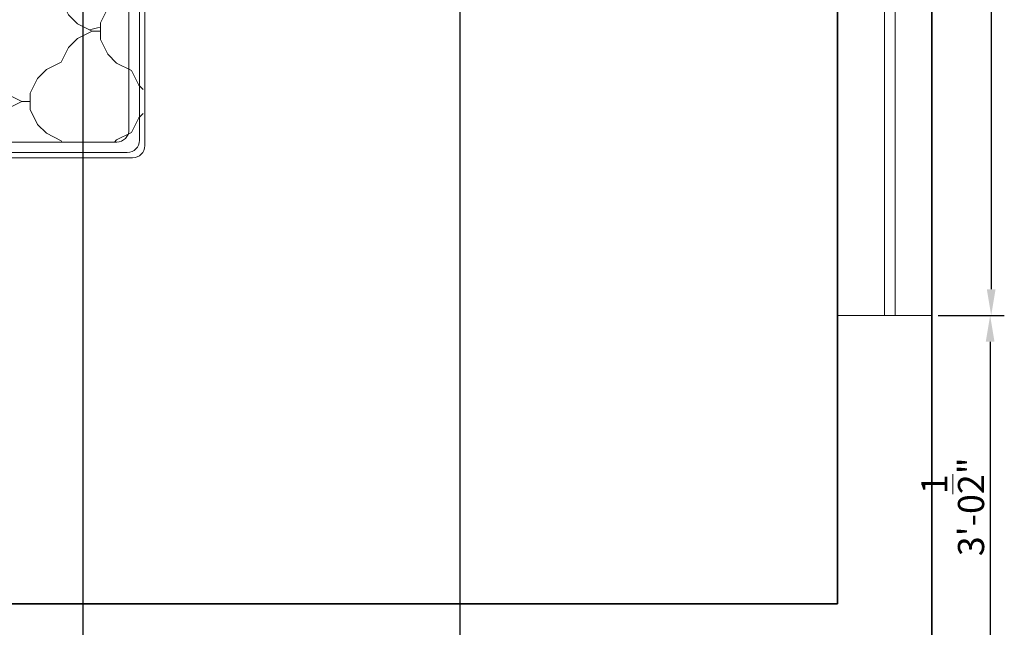
# Model space of a CAD drawing. Units: inches. Extents: x 1624 to 3956, y 1589 to 5028.
# Tile 5 of 16: x 2014 to 2108, y 2075 to 2133. Entities that reach past the tile are written whole.
import ezdxf

# ---------------------------------------------------------------- set-up
doc = ezdxf.new("R2010")
doc.units = ezdxf.units.IN
for name, color, linetype, lineweight in [('A-ANNO-DIMS', 2, 'Continuous', 13), ('A-FURN', 8, 'Continuous', 18), ('A-GLAZ', 4, 'Continuous', 18), ('A-WALL', 7, 'Continuous', 35)]:
    doc.layers.add(name, color=color, linetype=linetype, lineweight=lineweight)
doc.styles.get("Standard").update_dxf_attribs({"font": 'arial.ttf'})
doc.dimstyles.new('Copy of ISO-25', dxfattribs={"dimtxt": 2.5, "dimasz": 2.5, "dimexe": 1.25, "dimexo": 0.625, "dimtad": 1, "dimdec": 1, "dimlunit": 4, "dimtxsty": 'Standard', "dimcen": 2.5, "dimadec": 0, "dimazin": 0, "dimtfac": 1, "dimtdec": 1, "dimtmove": 0, "dimatfit": 3, "dimfxl": 1, "dimarcsym": 0})

# ---------------------------------------------------------------- blocks, each defined once
blk = doc.blocks.new('A$C029D5C69')
for p, q in [((0.4164, 2.0693), (0.4164, 2.0066)), ((2.2315, 2.0693), (0.4164, 2.0693)), ((2.2315, 2.0066), (2.2315, 2.0693)), ((0, 1.606), (0, 2.0066)), ((0, 2.0066), (0.505, 2.0066)), ((0.4164, 2.0066), (2.2315, 2.0066)), ((0.505, 2.0066), (0.505, 1.606)), ((0.5252, 0.0351), (0.5252, 2.0066)), ((0.5403, 0.0502), (0.5403, 2.0066)), ((0.5706, 0.0805), (0.5706, 2.0066)), ((0.6869, 1.966), (0.6666, 2.0066)), ((0.7072, 2.0066), (0.6869, 1.966)), ((1.0902, 1.966), (1.0699, 2.0066)), ((1.1106, 2.0066), (1.0902, 1.966)), ((2.1114, 2.0087), (2.1114, 0.0351)), ((2.6479, 2.0066), (2.1429, 2.0066)), ((2.1429, 2.0066), (2.1429, 1.606)), ((2.6479, 1.606), (2.6479, 2.0066)), ((0.0151, 1.6211), (0.0151, 1.9915)), ((0.0151, 1.9915), (0.4899, 1.9915)), ((0.4899, 1.9915), (0.4899, 1.6211)), ((1.8954, 1.9865), (1.3081, 1.9865)), ((2.6328, 1.9915), (2.158, 1.9915)), ((2.158, 1.9915), (2.158, 1.6211)), ((2.6328, 1.6211), (2.6328, 1.9915)), ((0.2689, 1.9609), (0.2689, 1.6764)), ((0.6869, 1.9425), (0.6869, 1.966)), ((0.6869, 1.9425), (0.6869, 1.966)), ((1.0902, 1.9425), (1.0902, 1.966)), ((1.0902, 1.9425), (1.0902, 1.966)), ((1.8954, 1.9713), (1.3339, 1.9713)), ((1.3849, 1.9713), (1.3656, 1.952)), ((1.3945, 1.9713), (1.3714, 1.9483)), ((1.4249, 1.945), (1.3986, 1.9713)), ((1.4288, 1.9507), (1.4081, 1.9713)), ((1.4476, 1.9507), (1.4288, 1.9507)), ((1.4476, 1.9507), (1.4664, 1.9507)), ((1.487, 1.9713), (1.4664, 1.9507)), ((1.4966, 1.9713), (1.4703, 1.945)), ((1.527, 1.945), (1.5007, 1.9713)), ((1.5309, 1.9507), (1.5102, 1.9713)), ((1.5497, 1.9507), (1.5309, 1.9507)), ((1.5497, 1.9507), (1.5685, 1.9507)), ((1.5891, 1.9713), (1.5685, 1.9507)), ((1.5987, 1.9713), (1.5724, 1.945)), ((1.6291, 1.945), (1.6028, 1.9713)), ((1.633, 1.9507), (1.6123, 1.9713)), ((1.6518, 1.9507), (1.633, 1.9507)), ((1.6518, 1.9507), (1.6706, 1.9507)), ((1.6912, 1.9713), (1.6706, 1.9507)), ((1.7008, 1.9713), (1.6745, 1.945)), ((1.7312, 1.945), (1.7049, 1.9713)), ((1.7351, 1.9507), (1.7144, 1.9713)), ((1.7539, 1.9507), (1.7351, 1.9507)), ((1.7539, 1.9507), (1.7727, 1.9507)), ((1.7933, 1.9713), (1.7727, 1.9507)), ((1.8029, 1.9713), (1.7766, 1.945)), ((1.8333, 1.945), (1.807, 1.9713)), ((1.8372, 1.9507), (1.8165, 1.9713)), ((1.856, 1.9507), (1.8372, 1.9507)), ((1.856, 1.9507), (1.8748, 1.9507)), ((1.8954, 1.9713), (1.8748, 1.9507)), ((1.9043, 1.9707), (1.8787, 1.945)), ((1.9354, 1.945), (1.9114, 1.969)), ((2.379, 1.9609), (2.379, 1.6764)), ((0.6634, 1.9425), (0.621, 1.9213)), ((0.6634, 1.9425), (0.621, 1.9213)), ((0.6869, 1.9425), (0.6634, 1.9425)), ((0.6869, 1.9425), (0.7104, 1.9425)), ((0.7528, 1.9213), (0.7104, 1.9425)), ((0.7528, 1.9213), (0.7104, 1.9425)), ((1.0668, 1.9425), (1.0244, 1.9213)), ((1.0668, 1.9425), (1.0244, 1.9213)), ((1.0902, 1.9425), (1.0668, 1.9425)), ((1.0902, 1.9425), (1.1137, 1.9425)), ((1.1561, 1.9213), (1.1137, 1.9425)), ((1.1561, 1.9213), (1.1137, 1.9425)), ((1.4249, 1.945), (1.4059, 1.926)), ((1.4288, 1.9394), (1.4116, 1.9222)), ((1.4288, 1.9393), (1.4476, 1.9393)), ((1.4664, 1.9393), (1.4476, 1.9393)), ((1.493, 1.9128), (1.4664, 1.9394)), ((1.4986, 1.9167), (1.4703, 1.945)), ((1.527, 1.945), (1.4986, 1.9167)), ((1.5309, 1.9394), (1.5043, 1.9128)), ((1.5309, 1.9393), (1.5497, 1.9393)), ((1.5685, 1.9393), (1.5497, 1.9393)), ((1.595, 1.9128), (1.5685, 1.9394)), ((1.6007, 1.9167), (1.5724, 1.945)), ((1.6291, 1.945), (1.6007, 1.9167)), ((1.633, 1.9394), (1.6064, 1.9128)), ((1.633, 1.9393), (1.6518, 1.9393)), ((1.6706, 1.9393), (1.6518, 1.9393)), ((1.6971, 1.9128), (1.6706, 1.9394)), ((1.7028, 1.9167), (1.6745, 1.945)), ((1.7312, 1.945), (1.7028, 1.9167)), ((1.7351, 1.9394), (1.7085, 1.9128)), ((1.7351, 1.9393), (1.7539, 1.9393)), ((1.7727, 1.9393), (1.7539, 1.9393)), ((1.7992, 1.9128), (1.7727, 1.9394)), ((1.8049, 1.9167), (1.7766, 1.945)), ((1.8333, 1.945), (1.8049, 1.9167)), ((1.8372, 1.9394), (1.8106, 1.9128)), ((1.8372, 1.9393), (1.856, 1.9393)), ((1.8748, 1.9393), (1.856, 1.9393)), ((1.9013, 1.9128), (1.8748, 1.9394)), ((1.907, 1.9167), (1.8787, 1.945)), ((1.9354, 1.945), (1.907, 1.9167)), ((1.9393, 1.9394), (1.9127, 1.9128)), ((1.9393, 1.9393), (1.9404, 1.9393)), ((1.9414, 1.688), (1.9414, 1.931)), ((1.9565, 1.688), (1.9565, 1.931)), ((0.5955, 1.8958), (0.5743, 1.8534)), ((0.621, 1.9213), (0.5955, 1.8958)), ((0.7783, 1.8958), (0.7528, 1.9213)), ((0.7995, 1.8534), (0.7783, 1.8958)), ((0.9989, 1.8958), (0.9777, 1.8534)), ((1.0243, 1.9213), (0.9988, 1.8958)), ((1.1816, 1.8958), (1.1561, 1.9213)), ((1.2028, 1.8534), (1.1816, 1.8958)), ((1.493, 1.8752), (1.493, 1.9128)), ((1.5043, 1.8752), (1.5043, 1.9128)), ((1.595, 1.8752), (1.595, 1.9128)), ((1.6064, 1.8752), (1.6064, 1.9128)), ((1.6971, 1.8752), (1.6971, 1.9128)), ((1.7085, 1.8752), (1.7085, 1.9128)), ((1.7992, 1.8752), (1.7992, 1.9128)), ((1.8106, 1.8752), (1.8106, 1.9128)), ((1.9013, 1.8752), (1.9013, 1.9128)), ((1.9127, 1.8752), (1.9127, 1.9128)), ((1.493, 1.8752), (1.4867, 1.869)), ((1.4986, 1.8713), (1.4922, 1.8648)), ((1.527, 1.8429), (1.4986, 1.8713)), ((1.5309, 1.8486), (1.5043, 1.8752)), ((1.595, 1.8752), (1.5685, 1.8486)), ((1.6007, 1.8713), (1.5724, 1.8429)), ((1.6291, 1.8429), (1.6007, 1.8713)), ((1.633, 1.8486), (1.6064, 1.8752)), ((1.6971, 1.8752), (1.6706, 1.8486)), ((1.7028, 1.8713), (1.6745, 1.8429)), ((1.7312, 1.8429), (1.7028, 1.8713)), ((1.7351, 1.8486), (1.7085, 1.8752)), ((1.7992, 1.8752), (1.7727, 1.8486)), ((1.8049, 1.8713), (1.7766, 1.8429)), ((1.8333, 1.8429), (1.8049, 1.8713)), ((1.8372, 1.8486), (1.8106, 1.8752)), ((1.9013, 1.8752), (1.8748, 1.8486)), ((1.907, 1.8713), (1.8787, 1.8429)), ((1.9354, 1.8429), (1.907, 1.8713)), ((1.9393, 1.8486), (1.9127, 1.8752)), ((0.5743, 1.8534), (0.5706, 1.8515)), ((0.5743, 1.8534), (0.5706, 1.8515)), ((0.8419, 1.8322), (0.7995, 1.8534)), ((0.8419, 1.8322), (0.7995, 1.8534)), ((0.9777, 1.8534), (0.9353, 1.8322)), ((0.9777, 1.8534), (0.9353, 1.8322)), ((1.2452, 1.8322), (1.2028, 1.8534)), ((1.2452, 1.8322), (1.2028, 1.8534)), ((1.527, 1.8429), (1.5242, 1.8401)), ((1.5309, 1.8373), (1.5295, 1.8359)), ((1.5497, 1.8486), (1.5309, 1.8486)), ((1.5309, 1.8373), (1.5497, 1.8373)), ((1.5497, 1.8486), (1.5685, 1.8486)), ((1.5685, 1.8373), (1.5497, 1.8373)), ((1.595, 1.8107), (1.5685, 1.8373)), ((1.6007, 1.8146), (1.5724, 1.8429)), ((1.6291, 1.8429), (1.6007, 1.8146)), ((1.633, 1.8373), (1.6064, 1.8107)), ((1.6518, 1.8486), (1.633, 1.8486)), ((1.633, 1.8373), (1.6518, 1.8373)), ((1.6518, 1.8486), (1.6706, 1.8486)), ((1.6706, 1.8373), (1.6518, 1.8373)), ((1.6971, 1.8107), (1.6706, 1.8373)), ((1.7028, 1.8146), (1.6745, 1.8429)), ((1.7312, 1.8429), (1.7028, 1.8146)), ((1.7351, 1.8373), (1.7085, 1.8107)), ((1.7539, 1.8486), (1.7351, 1.8486)), ((1.7351, 1.8373), (1.7539, 1.8373)), ((1.7539, 1.8486), (1.7727, 1.8486)), ((1.7727, 1.8373), (1.7539, 1.8373)), ((1.7992, 1.8107), (1.7727, 1.8373)), ((1.8049, 1.8146), (1.7766, 1.8429)), ((1.8333, 1.8429), (1.8049, 1.8146)), ((1.8372, 1.8373), (1.8106, 1.8107)), ((1.856, 1.8486), (1.8372, 1.8486)), ((1.8372, 1.8373), (1.856, 1.8373)), ((1.856, 1.8486), (1.8748, 1.8486)), ((1.8748, 1.8373), (1.856, 1.8373)), ((1.9013, 1.8107), (1.8748, 1.8373)), ((1.907, 1.8146), (1.8787, 1.8429)), ((1.9354, 1.8429), (1.907, 1.8146)), ((1.9393, 1.8373), (1.9127, 1.8107)), ((1.9414, 1.8486), (1.9393, 1.8486)), ((1.9393, 1.8373), (1.9414, 1.8373)), ((0.1267, 1.8186), (0.4111, 1.8186)), ((0.8674, 1.8067), (0.8419, 1.8322)), ((0.9352, 1.8322), (0.9097, 1.8067)), ((1.2707, 1.8067), (1.2452, 1.8322)), ((1.595, 1.7806), (1.595, 1.8107)), ((1.6064, 1.7731), (1.6064, 1.8107)), ((1.6971, 1.7731), (1.6971, 1.8107)), ((1.7085, 1.7731), (1.7085, 1.8107)), ((1.7992, 1.7731), (1.7992, 1.8107)), ((1.8106, 1.7731), (1.8106, 1.8107)), ((1.9013, 1.7731), (1.9013, 1.8107)), ((1.9127, 1.7731), (1.9127, 1.8107)), ((2.2367, 1.8186), (2.5212, 1.8186)), ((0.8886, 1.7643), (0.8674, 1.8067)), ((0.9098, 1.8067), (0.8886, 1.7643)), ((1.2919, 1.7643), (1.2707, 1.8067)), ((0.8886, 1.7408), (0.8886, 1.7643)), ((1.2981, 1.7768), (1.2919, 1.7643)), ((1.2919, 1.7519), (1.2919, 1.7643)), ((1.633, 1.7465), (1.6064, 1.7731)), ((1.6971, 1.7731), (1.6706, 1.7465)), ((1.7028, 1.7692), (1.6745, 1.7408)), ((1.7312, 1.7408), (1.7028, 1.7692)), ((1.7351, 1.7465), (1.7085, 1.7731)), ((1.7992, 1.7731), (1.7727, 1.7465)), ((1.8049, 1.7692), (1.7766, 1.7408)), ((1.8333, 1.7408), (1.8049, 1.7692)), ((1.8372, 1.7465), (1.8106, 1.7731)), ((1.9013, 1.7731), (1.8748, 1.7465)), ((1.907, 1.7692), (1.8787, 1.7408)), ((1.9354, 1.7408), (1.907, 1.7692)), ((1.9393, 1.7465), (1.9127, 1.7731)), ((0.8651, 1.7408), (0.8227, 1.7196)), ((0.8651, 1.7408), (0.8227, 1.7196)), ((0.912, 1.7408), (0.8651, 1.7408)), ((0.9544, 1.7196), (0.912, 1.7408)), ((0.9544, 1.7196), (0.912, 1.7408)), ((1.2684, 1.7408), (1.226, 1.7196)), ((1.2684, 1.7408), (1.226, 1.7196)), ((1.2885, 1.7408), (1.2684, 1.7408)), ((1.6518, 1.7465), (1.633, 1.7465)), ((1.6443, 1.7352), (1.6518, 1.7352)), ((1.6518, 1.7465), (1.6706, 1.7465)), ((1.6706, 1.7352), (1.6518, 1.7352)), ((1.6971, 1.7086), (1.6706, 1.7352)), ((1.7028, 1.7125), (1.6745, 1.7408)), ((1.7312, 1.7408), (1.7028, 1.7125)), ((1.7351, 1.7352), (1.7085, 1.7086)), ((1.7539, 1.7465), (1.7351, 1.7465)), ((1.7351, 1.7352), (1.7539, 1.7352)), ((1.7539, 1.7465), (1.7727, 1.7465)), ((1.7727, 1.7352), (1.7539, 1.7352)), ((1.7992, 1.7086), (1.7727, 1.7352)), ((1.8049, 1.7125), (1.7766, 1.7408)), ((1.8333, 1.7408), (1.8049, 1.7125)), ((1.8372, 1.7352), (1.8106, 1.7086)), ((1.856, 1.7465), (1.8372, 1.7465)), ((1.8372, 1.7352), (1.856, 1.7352)), ((1.856, 1.7465), (1.8748, 1.7465)), ((1.8748, 1.7352), (1.856, 1.7352)), ((1.9013, 1.7086), (1.8748, 1.7352)), ((1.907, 1.7125), (1.8787, 1.7408)), ((1.9354, 1.7408), (1.907, 1.7125)), ((1.9393, 1.7352), (1.9127, 1.7086)), ((1.9414, 1.7465), (1.9393, 1.7465)), ((1.9393, 1.7352), (1.9414, 1.7352)), ((0.5766, 1.6941), (0.5706, 1.7002)), ((0.8227, 1.7196), (0.7972, 1.6941)), ((0.98, 1.6941), (0.9545, 1.7196)), ((1.226, 1.7196), (1.2005, 1.6941)), ((1.6971, 1.682), (1.6971, 1.7086)), ((1.7085, 1.671), (1.7085, 1.7086)), ((1.7992, 1.671), (1.7992, 1.7086)), ((1.8106, 1.671), (1.8106, 1.7086)), ((1.9013, 1.671), (1.9013, 1.7086)), ((1.9127, 1.671), (1.9127, 1.7086)), ((2.5551, 1.6275), (2.5551, 1.696)), ((0.5978, 1.6517), (0.5766, 1.6941)), ((0.7972, 1.6941), (0.776, 1.6517)), ((1.0011, 1.6517), (0.9799, 1.6941)), ((1.2005, 1.6941), (1.1793, 1.6517)), ((1.7318, 1.6477), (1.7085, 1.671)), ((1.7992, 1.671), (1.7759, 1.6477)), ((1.8339, 1.6477), (1.8106, 1.671)), ((1.9013, 1.671), (1.878, 1.6477)), ((1.926, 1.6577), (1.9127, 1.671)), ((0.6402, 1.6305), (0.5978, 1.6517)), ((0.6402, 1.6305), (0.5978, 1.6517)), ((0.776, 1.6517), (0.7336, 1.6305)), ((0.776, 1.6517), (0.7336, 1.6305)), ((1.0435, 1.6305), (1.0011, 1.6517)), ((1.0435, 1.6305), (1.0011, 1.6517)), ((1.1793, 1.6517), (1.1369, 1.6305)), ((1.1793, 1.6517), (1.1369, 1.6305)), ((1.8961, 1.6477), (1.7289, 1.6477)), ((1.8049, 1.6671), (1.7855, 1.6477)), ((1.8244, 1.6477), (1.8049, 1.6671)), ((1.907, 1.6671), (1.8876, 1.6477)), ((1.9202, 1.6539), (1.907, 1.6671)), ((0.4899, 1.6211), (0.0151, 1.6211)), ((0.6657, 1.605), (0.6402, 1.6305)), ((0.7336, 1.6305), (0.7081, 1.605)), ((1.0691, 1.605), (1.0436, 1.6305)), ((1.1369, 1.6305), (1.1114, 1.605)), ((1.8961, 1.6325), (1.7422, 1.6325)), ((2.158, 1.6211), (2.6328, 1.6211)), ((0.505, 1.606), (0, 1.606)), ((0.6869, 1.5626), (0.6657, 1.605)), ((0.7081, 1.605), (0.6869, 1.5626)), ((1.0902, 1.5626), (1.069, 1.605)), ((1.1114, 1.605), (1.0902, 1.5626)), ((2.1429, 1.606), (2.6479, 1.606)), ((0.6869, 1.5392), (0.6869, 1.5626)), ((0.6869, 1.5392), (0.6869, 1.5626)), ((1.0902, 1.5392), (1.0902, 1.5626)), ((1.0902, 1.5392), (1.0902, 1.5626)), ((0.6634, 1.5391), (0.621, 1.5179)), ((0.6634, 1.5391), (0.621, 1.5179)), ((0.6869, 1.5392), (0.6634, 1.5392)), ((0.6869, 1.5392), (0.7104, 1.5392)), ((0.7528, 1.5179), (0.7104, 1.5391)), ((0.7528, 1.5179), (0.7104, 1.5391)), ((1.0668, 1.5391), (1.0244, 1.5179)), ((1.0668, 1.5391), (1.0244, 1.5179)), ((1.0902, 1.5392), (1.0668, 1.5392)), ((1.0902, 1.5392), (1.1137, 1.5392)), ((1.1561, 1.5179), (1.1137, 1.5391)), ((1.1561, 1.5179), (1.1137, 1.5391)), ((1.4534, 1.5308), (1.4277, 1.5179)), ((1.4534, 1.5308), (1.4277, 1.5179)), ((0.621, 1.5179), (0.5955, 1.4924)), ((0.7783, 1.4924), (0.7528, 1.5179)), ((1.0243, 1.5179), (0.9988, 1.4924)), ((1.1816, 1.4924), (1.1561, 1.5179)), ((1.4277, 1.5179), (1.4022, 1.4924)), ((0.5955, 1.4925), (0.5743, 1.4501)), ((0.7995, 1.4501), (0.7783, 1.4925)), ((0.9989, 1.4925), (0.9777, 1.4501)), ((1.2028, 1.4501), (1.1816, 1.4925)), ((1.4022, 1.4925), (1.381, 1.4501)), ((0.5743, 1.45), (0.5706, 1.4481)), ((0.5743, 1.45), (0.5706, 1.4481)), ((0.8419, 1.4288), (0.7995, 1.45)), ((0.8419, 1.4288), (0.7995, 1.45)), ((0.9777, 1.45), (0.9353, 1.4288)), ((0.9777, 1.45), (0.9353, 1.4288)), ((1.2452, 1.4288), (1.2028, 1.45)), ((1.2452, 1.4288), (1.2028, 1.45)), ((1.381, 1.45), (1.3386, 1.4288)), ((1.381, 1.45), (1.3386, 1.4288)), ((1.6062, 1.4501), (1.5966, 1.4692)), ((1.6486, 1.4288), (1.6062, 1.45)), ((1.6486, 1.4288), (1.6062, 1.45)), ((0.8674, 1.4033), (0.8419, 1.4288)), ((0.9352, 1.4288), (0.9097, 1.4033)), ((1.2707, 1.4033), (1.2452, 1.4288)), ((1.3386, 1.4288), (1.3131, 1.4033)), ((1.6741, 1.4033), (1.6486, 1.4288)), ((0.5403, 1.4117), (0.5706, 1.4117)), ((0.8886, 1.361), (0.8674, 1.4034)), ((0.9098, 1.4034), (0.8886, 1.361)), ((1.2919, 1.361), (1.2707, 1.4034)), ((1.3131, 1.4034), (1.2919, 1.361)), ((1.6953, 1.361), (1.6741, 1.4034)), ((1.714, 1.3984), (1.6953, 1.361)), ((0.8886, 1.3375), (0.8886, 1.3609)), ((1.2919, 1.3375), (1.2919, 1.3609)), ((1.6953, 1.3375), (1.6953, 1.3609)), ((0.8651, 1.3374), (0.8227, 1.3162)), ((0.8651, 1.3374), (0.8227, 1.3162)), ((0.912, 1.3375), (0.8651, 1.3375)), ((0.9544, 1.3162), (0.912, 1.3374)), ((0.9544, 1.3162), (0.912, 1.3374)), ((1.2684, 1.3374), (1.226, 1.3162)), ((1.2684, 1.3374), (1.226, 1.3162)), ((1.3154, 1.3375), (1.2684, 1.3375)), ((1.3578, 1.3162), (1.3154, 1.3374)), ((1.3578, 1.3162), (1.3154, 1.3374)), ((1.6718, 1.3374), (1.6294, 1.3162)), ((1.6718, 1.3374), (1.6294, 1.3162)), ((1.7187, 1.3375), (1.6718, 1.3375)), ((1.7611, 1.3162), (1.7187, 1.3374)), ((1.7611, 1.3162), (1.7187, 1.3374)), ((0.8227, 1.3163), (0.7972, 1.2908)), ((0.98, 1.2908), (0.9545, 1.3163)), ((1.226, 1.3163), (1.2005, 1.2908)), ((1.3833, 1.2908), (1.3578, 1.3163)), ((1.6294, 1.3163), (1.6039, 1.2908)), ((1.7867, 1.2908), (1.7611, 1.3163)), ((0.5766, 1.2908), (0.5706, 1.2968)), ((0.5978, 1.2484), (0.5766, 1.2908)), ((0.7972, 1.2908), (0.776, 1.2484)), ((1.0011, 1.2484), (0.9799, 1.2908)), ((1.2005, 1.2908), (1.1793, 1.2484)), ((1.4045, 1.2484), (1.3833, 1.2908)), ((1.6039, 1.2908), (1.5827, 1.2484)), ((1.8078, 1.2484), (1.7866, 1.2908)), ((0.6402, 1.2271), (0.5978, 1.2483)), ((0.6402, 1.2271), (0.5978, 1.2483)), ((0.776, 1.2483), (0.7336, 1.2271)), ((0.776, 1.2483), (0.7336, 1.2271)), ((1.0435, 1.2271), (1.0011, 1.2483)), ((1.0435, 1.2271), (1.0011, 1.2483)), ((1.1793, 1.2483), (1.1369, 1.2271)), ((1.1793, 1.2483), (1.1369, 1.2271)), ((1.4469, 1.2271), (1.4045, 1.2483)), ((1.4469, 1.2271), (1.4045, 1.2483)), ((1.5827, 1.2483), (1.5403, 1.2271)), ((1.5827, 1.2483), (1.5403, 1.2271)), ((1.8502, 1.2271), (1.8078, 1.2483)), ((1.8502, 1.2271), (1.8078, 1.2483)), ((0.6657, 1.2017), (0.6402, 1.2272)), ((0.7336, 1.2272), (0.7081, 1.2017)), ((1.0691, 1.2017), (1.0436, 1.2272)), ((1.1369, 1.2272), (1.1114, 1.2017)), ((1.4724, 1.2017), (1.4469, 1.2272)), ((1.5403, 1.2272), (1.5148, 1.2017)), ((1.8758, 1.2017), (1.8503, 1.2272)), ((0.5403, 1.21), (0.5706, 1.21)), ((0.6869, 1.1593), (0.6657, 1.2017)), ((0.7081, 1.2017), (0.6869, 1.1593)), ((1.0902, 1.1593), (1.069, 1.2017)), ((1.1114, 1.2017), (1.0902, 1.1593)), ((1.4936, 1.1593), (1.4724, 1.2017)), ((1.5148, 1.2017), (1.4936, 1.1593)), ((1.8969, 1.1593), (1.8757, 1.2017)), ((1.9181, 1.2017), (1.8969, 1.1593)), ((1.9215, 1.2051), (1.9181, 1.2017)), ((0.6869, 1.1358), (0.6869, 1.1593)), ((0.6869, 1.1358), (0.6869, 1.1593)), ((1.0902, 1.1358), (1.0902, 1.1593)), ((1.0902, 1.1358), (1.0902, 1.1593)), ((1.4936, 1.1358), (1.4936, 1.1593)), ((1.4936, 1.1358), (1.4936, 1.1593)), ((1.8969, 1.1358), (1.8969, 1.1593)), ((1.8969, 1.1358), (1.8969, 1.1593)), ((0.6634, 1.1358), (0.621, 1.1146)), ((0.6634, 1.1358), (0.621, 1.1146)), ((0.6869, 1.1358), (0.6634, 1.1358)), ((0.6869, 1.1358), (0.7104, 1.1358)), ((0.7528, 1.1146), (0.7104, 1.1358)), ((0.7528, 1.1146), (0.7104, 1.1358)), ((1.0668, 1.1358), (1.0244, 1.1146)), ((1.0668, 1.1358), (1.0244, 1.1146)), ((1.0902, 1.1358), (1.0668, 1.1358)), ((1.0902, 1.1358), (1.1137, 1.1358)), ((1.1561, 1.1146), (1.1137, 1.1358)), ((1.1561, 1.1146), (1.1137, 1.1358)), ((1.4701, 1.1358), (1.4277, 1.1146)), ((1.4701, 1.1358), (1.4277, 1.1146)), ((1.4936, 1.1358), (1.4701, 1.1358)), ((1.4936, 1.1358), (1.5171, 1.1358)), ((1.5595, 1.1146), (1.5171, 1.1358)), ((1.5595, 1.1146), (1.5171, 1.1358)), ((1.8735, 1.1358), (1.8311, 1.1146)), ((1.8735, 1.1358), (1.8311, 1.1146)), ((1.8969, 1.1358), (1.8735, 1.1358)), ((1.8969, 1.1358), (1.9204, 1.1358)), ((1.9628, 1.1146), (1.9204, 1.1358)), ((1.9628, 1.1146), (1.9204, 1.1358)), ((0.621, 1.1146), (0.5955, 1.0891)), ((0.7783, 1.0891), (0.7528, 1.1146)), ((1.0243, 1.1146), (0.9988, 1.0891)), ((1.1816, 1.0891), (1.1561, 1.1146)), ((1.4277, 1.1146), (1.4022, 1.0891)), ((1.585, 1.0891), (1.5595, 1.1146)), ((1.831, 1.1146), (1.8055, 1.0891)), ((1.9883, 1.0891), (1.9628, 1.1146)), ((0.5955, 1.0891), (0.5743, 1.0467)), ((0.7995, 1.0467), (0.7783, 1.0891)), ((0.9989, 1.0891), (0.9777, 1.0467)), ((1.2028, 1.0467), (1.1816, 1.0891)), ((1.4022, 1.0891), (1.381, 1.0467)), ((1.6062, 1.0467), (1.585, 1.0891)), ((1.8056, 1.0891), (1.7844, 1.0467)), ((2.0095, 1.0467), (1.9883, 1.0891)), ((0.5743, 1.0467), (0.5706, 1.0448)), ((0.5743, 1.0467), (0.5706, 1.0448)), ((0.8419, 1.0255), (0.7995, 1.0467)), ((0.8419, 1.0255), (0.7995, 1.0467)), ((0.9777, 1.0467), (0.9353, 1.0255)), ((0.9777, 1.0467), (0.9353, 1.0255)), ((1.2452, 1.0255), (1.2028, 1.0467)), ((1.2452, 1.0255), (1.2028, 1.0467)), ((1.381, 1.0467), (1.3386, 1.0255)), ((1.381, 1.0467), (1.3386, 1.0255)), ((1.6486, 1.0255), (1.6062, 1.0467)), ((1.6486, 1.0255), (1.6062, 1.0467)), ((1.7844, 1.0467), (1.742, 1.0255)), ((1.7844, 1.0467), (1.742, 1.0255)), ((2.0276, 1.0376), (2.0095, 1.0467)), ((2.0276, 1.0376), (2.0095, 1.0467)), ((0.8674, 1), (0.8419, 1.0255)), ((0.9352, 1.0255), (0.9097, 1)), ((1.2707, 1), (1.2452, 1.0255)), ((1.3386, 1.0255), (1.3131, 1)), ((1.6741, 1), (1.6486, 1.0255)), ((1.7419, 1.0255), (1.7164, 1)), ((0.8886, 0.9576), (0.8674, 1)), ((0.9098, 1), (0.8886, 0.9576)), ((1.2919, 0.9576), (1.2707, 1)), ((1.3131, 1), (1.2919, 0.9576)), ((1.6953, 0.9576), (1.6741, 1)), ((1.7165, 1), (1.6953, 0.9576)), ((0.8651, 0.9341), (0.8227, 0.9129)), ((0.8651, 0.9341), (0.8227, 0.9129)), ((0.912, 0.9341), (0.8651, 0.9341)), ((0.8886, 0.9341), (0.8886, 0.9576)), ((0.9544, 0.9129), (0.912, 0.9341)), ((0.9544, 0.9129), (0.912, 0.9341)), ((1.2684, 0.9341), (1.226, 0.9129)), ((1.2684, 0.9341), (1.226, 0.9129)), ((1.3154, 0.9341), (1.2684, 0.9341)), ((1.2919, 0.9341), (1.2919, 0.9576)), ((1.3578, 0.9129), (1.3154, 0.9341)), ((1.3578, 0.9129), (1.3154, 0.9341)), ((1.6718, 0.9341), (1.6294, 0.9129)), ((1.6718, 0.9341), (1.6294, 0.9129)), ((1.7187, 0.9341), (1.6718, 0.9341)), ((1.6953, 0.9341), (1.6953, 0.9576)), ((1.7611, 0.9129), (1.7187, 0.9341)), ((1.7611, 0.9129), (1.7187, 0.9341)), ((2.066, 0.9457), (2.066, 0.0805)), ((0.8227, 0.9129), (0.7972, 0.8874)), ((0.98, 0.8874), (0.9545, 0.9129)), ((1.226, 0.9129), (1.2005, 0.8874)), ((1.3833, 0.8874), (1.3578, 0.9129)), ((1.6294, 0.9129), (1.6039, 0.8874)), ((1.7867, 0.8874), (1.7611, 0.9129)), ((2.0327, 0.9129), (2.0072, 0.8874)), ((2.066, 0.9295), (2.0327, 0.9129)), ((2.066, 0.9295), (2.0327, 0.9129)), ((0.5766, 0.8874), (0.5706, 0.8935)), ((0.5978, 0.845), (0.5766, 0.8874)), ((0.7972, 0.8874), (0.776, 0.845)), ((1.0011, 0.845), (0.9799, 0.8874)), ((1.2005, 0.8874), (1.1793, 0.845)), ((1.4045, 0.845), (1.3833, 0.8874)), ((1.6039, 0.8874), (1.5827, 0.845)), ((1.8078, 0.845), (1.7866, 0.8874)), ((2.0072, 0.8874), (1.986, 0.845)), ((0.6402, 0.8238), (0.5978, 0.845)), ((0.6402, 0.8238), (0.5978, 0.845)), ((0.6657, 0.7983), (0.6402, 0.8238)), ((0.7336, 0.8238), (0.7081, 0.7983)), ((0.776, 0.845), (0.7336, 0.8238)), ((0.776, 0.845), (0.7336, 0.8238)), ((1.0435, 0.8238), (1.0011, 0.845)), ((1.0435, 0.8238), (1.0011, 0.845)), ((1.0691, 0.7983), (1.0436, 0.8238)), ((1.1369, 0.8238), (1.1114, 0.7983)), ((1.1793, 0.845), (1.1369, 0.8238)), ((1.1793, 0.845), (1.1369, 0.8238)), ((1.4469, 0.8238), (1.4045, 0.845)), ((1.4469, 0.8238), (1.4045, 0.845)), ((1.4724, 0.7983), (1.4469, 0.8238)), ((1.5403, 0.8238), (1.5148, 0.7983)), ((1.5827, 0.845), (1.5403, 0.8238)), ((1.5827, 0.845), (1.5403, 0.8238)), ((1.8502, 0.8238), (1.8078, 0.845)), ((1.8502, 0.8238), (1.8078, 0.845)), ((1.8758, 0.7983), (1.8503, 0.8238)), ((1.9436, 0.8238), (1.9181, 0.7983)), ((1.986, 0.845), (1.9436, 0.8238)), ((1.986, 0.845), (1.9436, 0.8238)), ((2.0962, 0.8369), (2.0962, 0.0502)), ((0.6869, 0.7559), (0.6657, 0.7983)), ((0.7081, 0.7983), (0.6869, 0.7559)), ((1.0902, 0.7559), (1.069, 0.7983)), ((1.1114, 0.7983), (1.0902, 0.7559)), ((1.4936, 0.7559), (1.4724, 0.7983)), ((1.5148, 0.7983), (1.4936, 0.7559)), ((1.8969, 0.7559), (1.8757, 0.7983)), ((1.9181, 0.7983), (1.8969, 0.7559)), ((0.6869, 0.7325), (0.6869, 0.7559)), ((0.6869, 0.7325), (0.6869, 0.7559)), ((1.0902, 0.7325), (1.0902, 0.7559)), ((1.0902, 0.7325), (1.0902, 0.7559)), ((1.2024, 0.7028), (1.2503, 0.7507)), ((1.4936, 0.7325), (1.4936, 0.7559)), ((1.4936, 0.7325), (1.4936, 0.7559)), ((1.8969, 0.7325), (1.8969, 0.7559)), ((1.8969, 0.7325), (1.8969, 0.7559)), ((0.621, 0.7113), (0.5955, 0.6858)), ((0.6634, 0.7324), (0.621, 0.7112)), ((0.6634, 0.7324), (0.621, 0.7112)), ((0.6869, 0.7325), (0.6634, 0.7325)), ((0.6869, 0.7325), (0.7104, 0.7325)), ((0.7528, 0.7112), (0.7104, 0.7324)), ((0.7528, 0.7112), (0.7104, 0.7324)), ((0.7783, 0.6858), (0.7528, 0.7113)), ((1.0243, 0.7113), (0.9988, 0.6858)), ((1.0668, 0.7324), (1.0244, 0.7112)), ((1.0668, 0.7324), (1.0244, 0.7112)), ((1.0902, 0.7325), (1.0668, 0.7325)), ((1.0902, 0.7325), (1.1137, 0.7325)), ((1.1561, 0.7112), (1.1137, 0.7324)), ((1.1561, 0.7112), (1.1137, 0.7324)), ((1.1816, 0.6858), (1.1561, 0.7113)), ((1.4277, 0.7113), (1.4022, 0.6858)), ((1.4701, 0.7324), (1.4277, 0.7112)), ((1.4701, 0.7324), (1.4277, 0.7112)), ((1.4936, 0.7325), (1.4701, 0.7325)), ((1.4936, 0.7325), (1.5171, 0.7325)), ((1.5595, 0.7112), (1.5171, 0.7324)), ((1.5595, 0.7112), (1.5171, 0.7324)), ((1.585, 0.6858), (1.5595, 0.7113)), ((1.831, 0.7113), (1.8055, 0.6858)), ((1.8735, 0.7324), (1.8311, 0.7112)), ((1.8735, 0.7324), (1.8311, 0.7112)), ((1.8969, 0.7325), (1.8735, 0.7325)), ((1.8969, 0.7325), (1.9204, 0.7325)), ((1.9628, 0.7112), (1.9204, 0.7324)), ((1.9628, 0.7112), (1.9204, 0.7324)), ((1.9883, 0.6858), (1.9628, 0.7113)), ((0.5955, 0.6858), (0.5743, 0.6434)), ((0.7995, 0.6434), (0.7783, 0.6858)), ((0.9989, 0.6858), (0.9777, 0.6434)), ((1.2028, 0.6434), (1.1816, 0.6858)), ((1.4022, 0.6858), (1.381, 0.6434)), ((1.6062, 0.6434), (1.585, 0.6858)), ((1.8056, 0.6858), (1.7844, 0.6434)), ((2.0095, 0.6434), (1.9883, 0.6858)), ((0.5743, 0.6433), (0.5706, 0.6414)), ((0.5743, 0.6433), (0.5706, 0.6414)), ((0.8419, 0.6221), (0.7995, 0.6433)), ((0.8419, 0.6221), (0.7995, 0.6433)), ((0.8674, 0.5967), (0.8419, 0.6222)), ((0.9352, 0.6222), (0.9097, 0.5967)), ((0.9777, 0.6433), (0.9353, 0.6221)), ((0.9777, 0.6433), (0.9353, 0.6221)), ((1.2452, 0.6221), (1.2028, 0.6433)), ((1.2452, 0.6221), (1.2028, 0.6433)), ((1.2707, 0.5967), (1.2452, 0.6222)), ((1.3386, 0.6222), (1.3131, 0.5967)), ((1.381, 0.6433), (1.3386, 0.6221)), ((1.381, 0.6433), (1.3386, 0.6221)), ((1.6486, 0.6221), (1.6062, 0.6433)), ((1.6486, 0.6221), (1.6062, 0.6433)), ((1.6741, 0.5967), (1.6486, 0.6222)), ((1.7419, 0.6222), (1.7164, 0.5967)), ((1.7844, 0.6433), (1.742, 0.6221)), ((1.7844, 0.6433), (1.742, 0.6221)), ((2.0519, 0.6221), (2.0095, 0.6433)), ((2.0519, 0.6221), (2.0095, 0.6433)), ((2.066, 0.6081), (2.0519, 0.6222)), ((0.8886, 0.5543), (0.8674, 0.5967)), ((0.9098, 0.5967), (0.8886, 0.5543)), ((1.2919, 0.5543), (1.2707, 0.5967)), ((1.3131, 0.5967), (1.2919, 0.5543)), ((1.6953, 0.5543), (1.6741, 0.5967)), ((1.7165, 0.5967), (1.6953, 0.5543)), ((0.8886, 0.5308), (0.8886, 0.5543)), ((1.2919, 0.5308), (1.2919, 0.5543)), ((1.6953, 0.5308), (1.6953, 0.5543)), ((0.8227, 0.5096), (0.7972, 0.4841)), ((0.8651, 0.5308), (0.8227, 0.5096)), ((0.8651, 0.5308), (0.8227, 0.5096)), ((0.912, 0.5308), (0.8651, 0.5308)), ((0.9544, 0.5096), (0.912, 0.5308)), ((0.9544, 0.5096), (0.912, 0.5308)), ((0.98, 0.4841), (0.9545, 0.5096)), ((1.226, 0.5096), (1.2005, 0.4841)), ((1.2684, 0.5308), (1.226, 0.5096)), ((1.2684, 0.5308), (1.226, 0.5096)), ((1.3154, 0.5308), (1.2684, 0.5308)), ((1.3578, 0.5096), (1.3154, 0.5308)), ((1.3578, 0.5096), (1.3154, 0.5308)), ((1.3833, 0.4841), (1.3578, 0.5096)), ((1.6294, 0.5096), (1.6039, 0.4841)), ((1.6718, 0.5308), (1.6294, 0.5096)), ((1.6718, 0.5308), (1.6294, 0.5096)), ((1.7187, 0.5308), (1.6718, 0.5308)), ((1.7611, 0.5096), (1.7187, 0.5308)), ((1.7611, 0.5096), (1.7187, 0.5308)), ((1.7867, 0.4841), (1.7611, 0.5096)), ((2.0327, 0.5096), (2.0072, 0.4841)), ((2.066, 0.5262), (2.0327, 0.5096)), ((2.066, 0.5262), (2.0327, 0.5096)), ((0.5766, 0.4841), (0.5706, 0.4901)), ((0.5978, 0.4417), (0.5766, 0.4841)), ((0.7972, 0.4841), (0.776, 0.4417)), ((1.0011, 0.4417), (0.9799, 0.4841)), ((1.2005, 0.4841), (1.1793, 0.4417)), ((1.4045, 0.4417), (1.3833, 0.4841)), ((1.6039, 0.4841), (1.5827, 0.4417)), ((1.8078, 0.4417), (1.7866, 0.4841)), ((2.0072, 0.4841), (1.986, 0.4417)), ((0.6402, 0.4205), (0.5978, 0.4417)), ((0.6402, 0.4205), (0.5978, 0.4417)), ((0.776, 0.4417), (0.7336, 0.4205)), ((0.776, 0.4417), (0.7336, 0.4205)), ((1.0435, 0.4205), (1.0011, 0.4417)), ((1.0435, 0.4205), (1.0011, 0.4417)), ((1.1793, 0.4417), (1.1369, 0.4205)), ((1.1793, 0.4417), (1.1369, 0.4205)), ((1.4469, 0.4205), (1.4045, 0.4417)), ((1.4469, 0.4205), (1.4045, 0.4417)), ((1.5827, 0.4417), (1.5403, 0.4205)), ((1.5827, 0.4417), (1.5403, 0.4205)), ((1.8502, 0.4205), (1.8078, 0.4417)), ((1.8502, 0.4205), (1.8078, 0.4417)), ((1.986, 0.4417), (1.9436, 0.4205)), ((1.986, 0.4417), (1.9436, 0.4205)), ((0.6657, 0.395), (0.6402, 0.4205)), ((0.7336, 0.4205), (0.7081, 0.395)), ((1.0691, 0.395), (1.0436, 0.4205)), ((1.1369, 0.4205), (1.1114, 0.395)), ((1.4724, 0.395), (1.4469, 0.4205)), ((1.5403, 0.4205), (1.5148, 0.395)), ((1.8758, 0.395), (1.8503, 0.4205)), ((1.9436, 0.4205), (1.9181, 0.395)), ((0.6869, 0.3526), (0.6657, 0.395)), ((0.7081, 0.395), (0.6869, 0.3526)), ((1.0902, 0.3526), (1.069, 0.395)), ((1.1114, 0.395), (1.0902, 0.3526)), ((1.4936, 0.3526), (1.4724, 0.395)), ((1.5148, 0.395), (1.4936, 0.3526)), ((1.8969, 0.3526), (1.8757, 0.395)), ((1.9181, 0.395), (1.8969, 0.3526)), ((0.6869, 0.3291), (0.6869, 0.3526)), ((0.6869, 0.3291), (0.6869, 0.3526)), ((1.0902, 0.3291), (1.0902, 0.3526)), ((1.0902, 0.3291), (1.0902, 0.3526)), ((1.4936, 0.3291), (1.4936, 0.3526)), ((1.4936, 0.3291), (1.4936, 0.3526)), ((1.8969, 0.3291), (1.8969, 0.3526)), ((1.8969, 0.3291), (1.8969, 0.3526)), ((0.6634, 0.3291), (0.621, 0.3079)), ((0.6634, 0.3291), (0.621, 0.3079)), ((0.6869, 0.3291), (0.6634, 0.3291)), ((0.6869, 0.3291), (0.7104, 0.3291)), ((0.7528, 0.3079), (0.7104, 0.3291)), ((0.7528, 0.3079), (0.7104, 0.3291)), ((1.0668, 0.3291), (1.0244, 0.3079)), ((1.0668, 0.3291), (1.0244, 0.3079)), ((1.0902, 0.3291), (1.0668, 0.3291)), ((1.0902, 0.3291), (1.1137, 0.3291)), ((1.1561, 0.3079), (1.1137, 0.3291)), ((1.1561, 0.3079), (1.1137, 0.3291)), ((1.4701, 0.3291), (1.4277, 0.3079)), ((1.4701, 0.3291), (1.4277, 0.3079)), ((1.4936, 0.3291), (1.4701, 0.3291)), ((1.4936, 0.3291), (1.5171, 0.3291)), ((1.5595, 0.3079), (1.5171, 0.3291)), ((1.5595, 0.3079), (1.5171, 0.3291)), ((1.8735, 0.3291), (1.8311, 0.3079)), ((1.8735, 0.3291), (1.8311, 0.3079)), ((1.8969, 0.3291), (1.8735, 0.3291)), ((1.8969, 0.3291), (1.9204, 0.3291)), ((1.9628, 0.3079), (1.9204, 0.3291)), ((1.9628, 0.3079), (1.9204, 0.3291)), ((0.621, 0.3079), (0.5955, 0.2824)), ((0.7783, 0.2824), (0.7528, 0.3079)), ((1.0243, 0.3079), (0.9988, 0.2824)), ((1.1816, 0.2824), (1.1561, 0.3079)), ((1.4277, 0.3079), (1.4022, 0.2824)), ((1.585, 0.2824), (1.5595, 0.3079)), ((1.831, 0.3079), (1.8055, 0.2824)), ((1.9883, 0.2824), (1.9628, 0.3079)), ((0.5955, 0.2824), (0.5743, 0.24)), ((0.7995, 0.24), (0.7783, 0.2824)), ((0.9989, 0.2824), (0.9777, 0.24)), ((1.2028, 0.24), (1.1816, 0.2824)), ((1.4022, 0.2824), (1.381, 0.24)), ((1.6062, 0.24), (1.585, 0.2824)), ((1.8056, 0.2824), (1.7844, 0.24)), ((2.0095, 0.24), (1.9883, 0.2824)), ((0.5743, 0.24), (0.5706, 0.2381)), ((0.5743, 0.24), (0.5706, 0.2381)), ((0.8419, 0.2188), (0.7995, 0.24)), ((0.8419, 0.2188), (0.7995, 0.24)), ((0.9777, 0.24), (0.9353, 0.2188)), ((0.9777, 0.24), (0.9353, 0.2188)), ((1.2452, 0.2188), (1.2028, 0.24)), ((1.2452, 0.2188), (1.2028, 0.24)), ((1.381, 0.24), (1.3386, 0.2188)), ((1.381, 0.24), (1.3386, 0.2188)), ((1.6486, 0.2188), (1.6062, 0.24)), ((1.6486, 0.2188), (1.6062, 0.24)), ((1.7844, 0.24), (1.742, 0.2188)), ((1.7844, 0.24), (1.742, 0.2188)), ((2.0519, 0.2188), (2.0095, 0.24)), ((2.0519, 0.2188), (2.0095, 0.24)), ((0.8674, 0.1933), (0.8419, 0.2188)), ((0.9352, 0.2188), (0.9097, 0.1933)), ((1.2707, 0.1933), (1.2452, 0.2188)), ((1.3386, 0.2188), (1.3131, 0.1933)), ((1.6741, 0.1933), (1.6486, 0.2188)), ((1.7419, 0.2188), (1.7164, 0.1933)), ((2.066, 0.2047), (2.0519, 0.2188)), ((0.8886, 0.1509), (0.8674, 0.1933)), ((0.9098, 0.1933), (0.8886, 0.1509)), ((1.2919, 0.1509), (1.2707, 0.1933)), ((1.3131, 0.1933), (1.2919, 0.1509)), ((1.6953, 0.1509), (1.6741, 0.1933)), ((1.7165, 0.1933), (1.6953, 0.1509)), ((0.8886, 0.1275), (0.8886, 0.1509)), ((1.2919, 0.1275), (1.2919, 0.1509)), ((1.6953, 0.1275), (1.6953, 0.1509)), ((0.8651, 0.1274), (0.8227, 0.1062)), ((0.8651, 0.1274), (0.8227, 0.1062)), ((0.912, 0.1275), (0.8651, 0.1275)), ((0.9544, 0.1062), (0.912, 0.1274)), ((0.9544, 0.1062), (0.912, 0.1274)), ((1.2684, 0.1274), (1.226, 0.1062)), ((1.2684, 0.1274), (1.226, 0.1062)), ((1.3154, 0.1275), (1.2684, 0.1275)), ((1.3578, 0.1062), (1.3154, 0.1274)), ((1.3578, 0.1062), (1.3154, 0.1274)), ((1.6718, 0.1274), (1.6294, 0.1062)), ((1.6718, 0.1274), (1.6294, 0.1062)), ((1.7187, 0.1275), (1.6718, 0.1275)), ((1.7611, 0.1062), (1.7187, 0.1274)), ((1.7611, 0.1062), (1.7187, 0.1274)), ((2.066, 0.1228), (2.0327, 0.1062)), ((2.066, 0.1228), (2.0327, 0.1062)), ((0.5766, 0.0807), (0.5706, 0.0868)), ((0.8227, 0.1062), (0.7972, 0.0807)), ((0.98, 0.0807), (0.9545, 0.1062)), ((1.226, 0.1062), (1.2005, 0.0807)), ((1.3833, 0.0807), (1.3578, 0.1062)), ((1.6294, 0.1062), (1.6039, 0.0807)), ((1.7867, 0.0807), (1.7611, 0.1062)), ((2.0327, 0.1062), (2.0072, 0.0807)), ((0.5978, 0.0384), (0.5766, 0.0808)), ((0.7972, 0.0808), (0.776, 0.0384)), ((1.0011, 0.0384), (0.9799, 0.0808)), ((1.2005, 0.0808), (1.1793, 0.0384)), ((1.4045, 0.0384), (1.3833, 0.0808)), ((1.6039, 0.0808), (1.5827, 0.0384)), ((1.8078, 0.0384), (1.7866, 0.0808)), ((2.0072, 0.0808), (1.986, 0.0384)), ((0.6402, 0.0171), (0.5978, 0.0383)), ((0.6402, 0.0171), (0.5978, 0.0383)), ((2.0309, 0.0454), (0.6056, 0.0454)), ((0.776, 0.0383), (0.7336, 0.0171)), ((0.776, 0.0383), (0.7336, 0.0171)), ((1.0435, 0.0171), (1.0011, 0.0383)), ((1.0435, 0.0171), (1.0011, 0.0383)), ((1.1793, 0.0383), (1.1369, 0.0171)), ((1.1793, 0.0383), (1.1369, 0.0171)), ((1.4469, 0.0171), (1.4045, 0.0383)), ((1.4469, 0.0171), (1.4045, 0.0383)), ((1.5827, 0.0383), (1.5403, 0.0171)), ((1.5827, 0.0383), (1.5403, 0.0171)), ((1.8502, 0.0171), (1.8078, 0.0383)), ((1.8502, 0.0171), (1.8078, 0.0383)), ((1.986, 0.0383), (1.9436, 0.0171)), ((1.986, 0.0383), (1.9436, 0.0171)), ((2.0763, 0), (0.5603, 0)), ((2.0612, 0.0151), (0.5754, 0.0151)), ((0.6523, 0.005), (0.6402, 0.0171)), ((0.7336, 0.0171), (0.7215, 0.005)), ((1.0557, 0.005), (1.0436, 0.0171)), ((1.1369, 0.0171), (1.1248, 0.005)), ((1.459, 0.005), (1.4469, 0.0171)), ((1.5403, 0.0171), (1.5282, 0.005)), ((1.8623, 0.005), (1.8503, 0.0171)), ((1.9436, 0.0171), (1.9315, 0.005))]:
    blk.add_line(p, q)
at = {"ltscale": 0.005}
for p, q in [((0.4899, 1.6568), (0.0151, 1.9915)), ((0.0151, 1.6568), (0.4899, 1.9915)), ((2.6328, 1.6568), (2.158, 1.9915)), ((2.158, 1.6568), (2.6328, 1.9915)), ((0.0151, 1.6568), (0.4899, 1.6568)), ((2.6328, 1.6568), (2.158, 1.6568))]:
    blk.add_line(p, q, dxfattribs=at)
for centre, radius in [((0.2689, 1.8186), 0.1191), ((2.379, 1.8186), 0.1191), ((0.2689, 1.8186), 0.0711), ((2.379, 1.8186), 0.0711)]:
    blk.add_circle(centre, radius)
for centre, radius, start, end in [((0.2843, 0.0157), 0.6251, 10.2961, 13.2684), ((0.6056, 0.0805), 0.0351, 180, 270), ((2.0309, 0.0805), 0.0351, 270, 0), ((0.5603, 0.0351), 0.0351, 180, 270), ((0.5754, 0.0502), 0.0351, 180, 270), ((2.0612, 0.0502), 0.0351, 270, 0), ((2.0763, 0.0351), 0.0351, 270, 0)]:
    blk.add_arc(centre, radius, start, end)
for centre, major_axis, ratio, start_param, end_param in [((0.8506, 1.8527), (-0.4556, 0), 0.89, 2.430919, 3.53111), ((0.3667, 0.6698), (1.7398, 0.1668), 0.88072, -0.045073, 0.941433), ((1.8961, 1.931), (-0.0453, 0), 0.89, 3.141593, 4.712389), ((1.8961, 1.688), (-0.0453, 0), 0.89, 1.570796, 3.141593), ((1.0874, 0.6748), (1.021, 0.1213), 0.889348, -0.031673, 1.359628)]:
    blk.add_ellipse(centre, major_axis=major_axis, ratio=ratio, start_param=start_param, end_param=end_param)
for points, knots in [([(1.9565, 1.931), (1.9565, 1.9336), (1.9563, 1.9362), (1.9553, 1.9428), (1.9543, 1.9467), (1.9512, 1.9541), (1.9493, 1.9577), (1.9446, 1.9643), (1.942, 1.9674), (1.936, 1.9729), (1.9327, 1.9753), (1.9257, 1.9795), (1.922, 1.9813), (1.9142, 1.9841), (1.9102, 1.9851), (1.9028, 1.9862), (1.8995, 1.9865), (1.8961, 1.9865)], [3.141593, 3.141593, 3.141593, 3.141593, 3.277614, 3.277614, 3.488082, 3.488082, 3.698551, 3.698551, 3.909019, 3.909019, 4.119488, 4.119488, 4.329956, 4.329956, 4.540424, 4.540424, 4.712389, 4.712389, 4.712389, 4.712389]), ([(1.8961, 1.6325), (1.899, 1.6325), (1.9019, 1.6327), (1.9101, 1.6338), (1.9153, 1.6352), (1.9253, 1.6392), (1.93, 1.6418), (1.9385, 1.6481), (1.9423, 1.6519), (1.9481, 1.6594), (1.9503, 1.663), (1.9537, 1.6707), (1.955, 1.6747), (1.9563, 1.6818), (1.9565, 1.6849), (1.9565, 1.688)], [1.570796, 1.570796, 1.570796, 1.570796, 1.718836, 1.718836, 1.993452, 1.993452, 2.268068, 2.268068, 2.542684, 2.542684, 2.761386, 2.761386, 2.980087, 2.980087, 3.141593, 3.141593, 3.141593, 3.141593])]:
    blk.add_open_spline(points, degree=3, knots=knots)
blk = doc.blocks.new('A$C0D3A6DFA')
blk.add_blockref('A$C029D5C69', (0, 0))
blk = doc.blocks.new('*D40')
at = {"layer": 'A-ANNO-DIMS', "color": 0, "lineweight": -2, "transparency": 16777216}
for p, q in [((2101.204, 2176.795), (2107.51, 2176.795)), ((2106.26, 2174.295), (2106.26, 2107.295)), ((2101.204, 2104.795), (2107.51, 2104.795))]:
    blk.add_line(p, q, dxfattribs=at)
at = {"layer": 'A-ANNO-DIMS', "color": 0, "transparency": 16777216}
for points in [[(2105.843, 2174.295), (2106.676, 2174.295), (2106.26, 2176.795)], [(2105.843, 2107.295), (2106.676, 2107.295), (2106.26, 2104.795)]]:
    blk.add_solid(points, dxfattribs=at)
at = {"layer": 'Defpoints', "color": 0, "transparency": 16777216}
for p in [(2100.579, 2176.795), (2100.579, 2104.795), (2106.26, 2104.795)]:
    blk.add_point(p, dxfattribs=at)
at = {"layer": 'A-ANNO-DIMS', "color": 0, "transparency": 16777216, "insert": (2104.358, 2140.795), "char_height": 2.5, "attachment_point": 5, "rotation": 90}
blk.add_mtext("6'", dxfattribs=at)
blk = doc.blocks.new('*D41')
at = {"layer": 'A-ANNO-DIMS', "color": 0, "lineweight": -2, "transparency": 16777216}
for p, q in [((2101.204, 2104.795), (2107.407, 2104.795)), ((2106.157, 2102.295), (2106.157, 2070.795)), ((2101.204, 2068.295), (2107.407, 2068.295))]:
    blk.add_line(p, q, dxfattribs=at)
at = {"layer": 'A-ANNO-DIMS', "color": 0, "transparency": 16777216}
for points in [[(2105.74, 2102.295), (2106.574, 2102.295), (2106.157, 2104.795)], [(2105.74, 2070.795), (2106.574, 2070.795), (2106.157, 2068.295)]]:
    blk.add_solid(points, dxfattribs=at)
at = {"layer": 'Defpoints', "color": 0, "transparency": 16777216}
for p in [(2100.579, 2104.795), (2100.579, 2068.295), (2106.157, 2068.295)]:
    blk.add_point(p, dxfattribs=at)
at = {"layer": 'A-ANNO-DIMS', "color": 0, "transparency": 16777216, "insert": (2102.583, 2086.545), "char_height": 2.5, "attachment_point": 5, "rotation": 90}
blk.add_mtext('3\'-0{\\H1x;\\S1/2;}"', dxfattribs=at)
blk = doc.blocks.new('WINDOW-72IN')
for p, q in [((0, 9), (0, 0)), ((72, 0), (72, 9)), ((0, 4.5), (72, 4.5)), ((0, 3.5), (72, 3.5))]:
    blk.add_line(p, q)
blk = doc.blocks.new('*D90')
at = {"layer": 'A-ANNO-DIMS', "color": 0, "lineweight": -2, "transparency": 16777216}
for p, q in [((2019.579, 1941.92), (2019.579, 2612.845)), ((2055.579, 1941.92), (2055.579, 2612.845)), ((2022.079, 2611.595), (2053.079, 2611.595))]:
    blk.add_line(p, q, dxfattribs=at)
at = {"layer": 'A-ANNO-DIMS', "color": 0, "transparency": 16777216}
for points in [[(2022.079, 2612.011), (2022.079, 2611.178), (2019.579, 2611.595)], [(2053.079, 2612.011), (2053.079, 2611.178), (2055.579, 2611.595)]]:
    blk.add_solid(points, dxfattribs=at)
at = {"layer": 'Defpoints', "color": 0, "transparency": 16777216}
for p in [(2055.579, 2611.595), (2019.579, 1941.295), (2055.579, 1941.295)]:
    blk.add_point(p, dxfattribs=at)
at = {"layer": 'A-ANNO-DIMS', "color": 0, "transparency": 16777216, "insert": (2037.579, 2613.497), "char_height": 2.5, "attachment_point": 5}
blk.add_mtext('3\'-0"', dxfattribs=at)
blk = doc.blocks.new('*D98')
at = {"layer": 'A-ANNO-DIMS', "color": 0, "lineweight": -2, "transparency": 16777216}
for p, q in [((2090.954, 2245.295), (1628.859, 2245.295)), ((1630.109, 2079.795), (1630.109, 2242.795)), ((2090.954, 2077.295), (1628.859, 2077.295))]:
    blk.add_line(p, q, dxfattribs=at)
at = {"layer": 'A-ANNO-DIMS', "color": 0, "transparency": 16777216}
for points in [[(1629.692, 2242.795), (1630.525, 2242.795), (1630.109, 2245.295)], [(1629.692, 2079.795), (1630.525, 2079.795), (1630.109, 2077.295)]]:
    blk.add_solid(points, dxfattribs=at)
at = {"layer": 'Defpoints', "color": 0, "transparency": 16777216}
for p in [(1630.109, 2245.295), (2091.579, 2245.295), (2091.579, 2077.295)]:
    blk.add_point(p, dxfattribs=at)
at = {"layer": 'A-ANNO-DIMS', "color": 0, "transparency": 16777216, "insert": (1628.207, 2161.295), "char_height": 2.5, "attachment_point": 5, "rotation": 90}
blk.add_mtext('14\'-0"', dxfattribs=at)

msp = doc.modelspace()

# ---------------------------------------------------------------- linework, layer by layer
at = {"layer": 'A-GLAZ'}
msp.add_line((2100.579, 2176.795), (2100.579, 2104.795), dxfattribs=at)
at = {"layer": 'A-WALL'}
for p, q in [((2091.579, 2077.295), (2091.579, 2245.295)), ((2100.579, 2245.295), (2100.579, 2077.295)), ((2100.579, 2161.295), (2100.579, 2033.295)), ((2091.579, 2077.295), (1951.579, 2077.295)), ((2100.579, 2077.295), (2100.579, 2072.795)), ((2100.579, 2077.295), (2100.579, 2072.795))]:
    msp.add_line(p, q, dxfattribs=at)

# ---------------------------------------------------------------- block references
at = {"layer": 'A-FURN', "xscale": 33.26127928322124, "yscale": 33.26127928322124, "zscale": 33.26127928322124, "rotation": 90}
msp.add_blockref('A$C0D3A6DFA', (2025.461, 2102.371), dxfattribs=at)
at = {"layer": 'A-GLAZ', "rotation": 90.00000000000003}
msp.add_blockref('WINDOW-72IN', (2100.579, 2104.795), dxfattribs=at)

# ---------------------------------------------------------------- dimensions: what is measured, and where the dimension line sits
at = {"layer": 'A-ANNO-DIMS'}
dim = msp.add_linear_dim(base=(2055.579, 2611.595), p1=(2019.579, 1941.295), p2=(2055.579, 1941.295), dimstyle='Copy of ISO-25', override={"dimdec": 1, "dimlfac": 1, "dimrnd": 0, "dimzin": 1, "dimdsep": 46, "dimlunit": 4, "dimfrac": 2}, dxfattribs=at)
dim.commit()
dim.dimension.update_dxf_attribs({"geometry": '*D90', "text_midpoint": (2037.579, 2613.497)})
for base, p1, p2, override, picture, middle in [((1630.109, 2245.295), (2091.579, 2077.295), (2091.579, 2245.295), {"dimdec": 1, "dimlfac": 1, "dimrnd": 0, "dimzin": 1, "dimdsep": 46, "dimlunit": 4, "dimfrac": 2}, '*D98', (1628.207, 2161.295)), ((2106.26, 2104.795), (2100.579, 2176.795), (2100.579, 2104.795), {"dimclrd": 0, "dimclre": 0, "dimclrt": 0}, '*D40', (2104.358, 2140.795)), ((2106.157, 2068.295), (2100.579, 2104.795), (2100.579, 2068.295), {"dimclrd": 0, "dimclre": 0, "dimclrt": 0}, '*D41', (2102.583, 2086.545))]:
    dim = msp.add_linear_dim(base=base, p1=p1, p2=p2, angle=90, dimstyle='Copy of ISO-25', override=override, dxfattribs=at)
    dim.commit()
    dim.dimension.update_dxf_attribs({"geometry": picture, "text_midpoint": middle})

doc.saveas('drawing.dxf')
